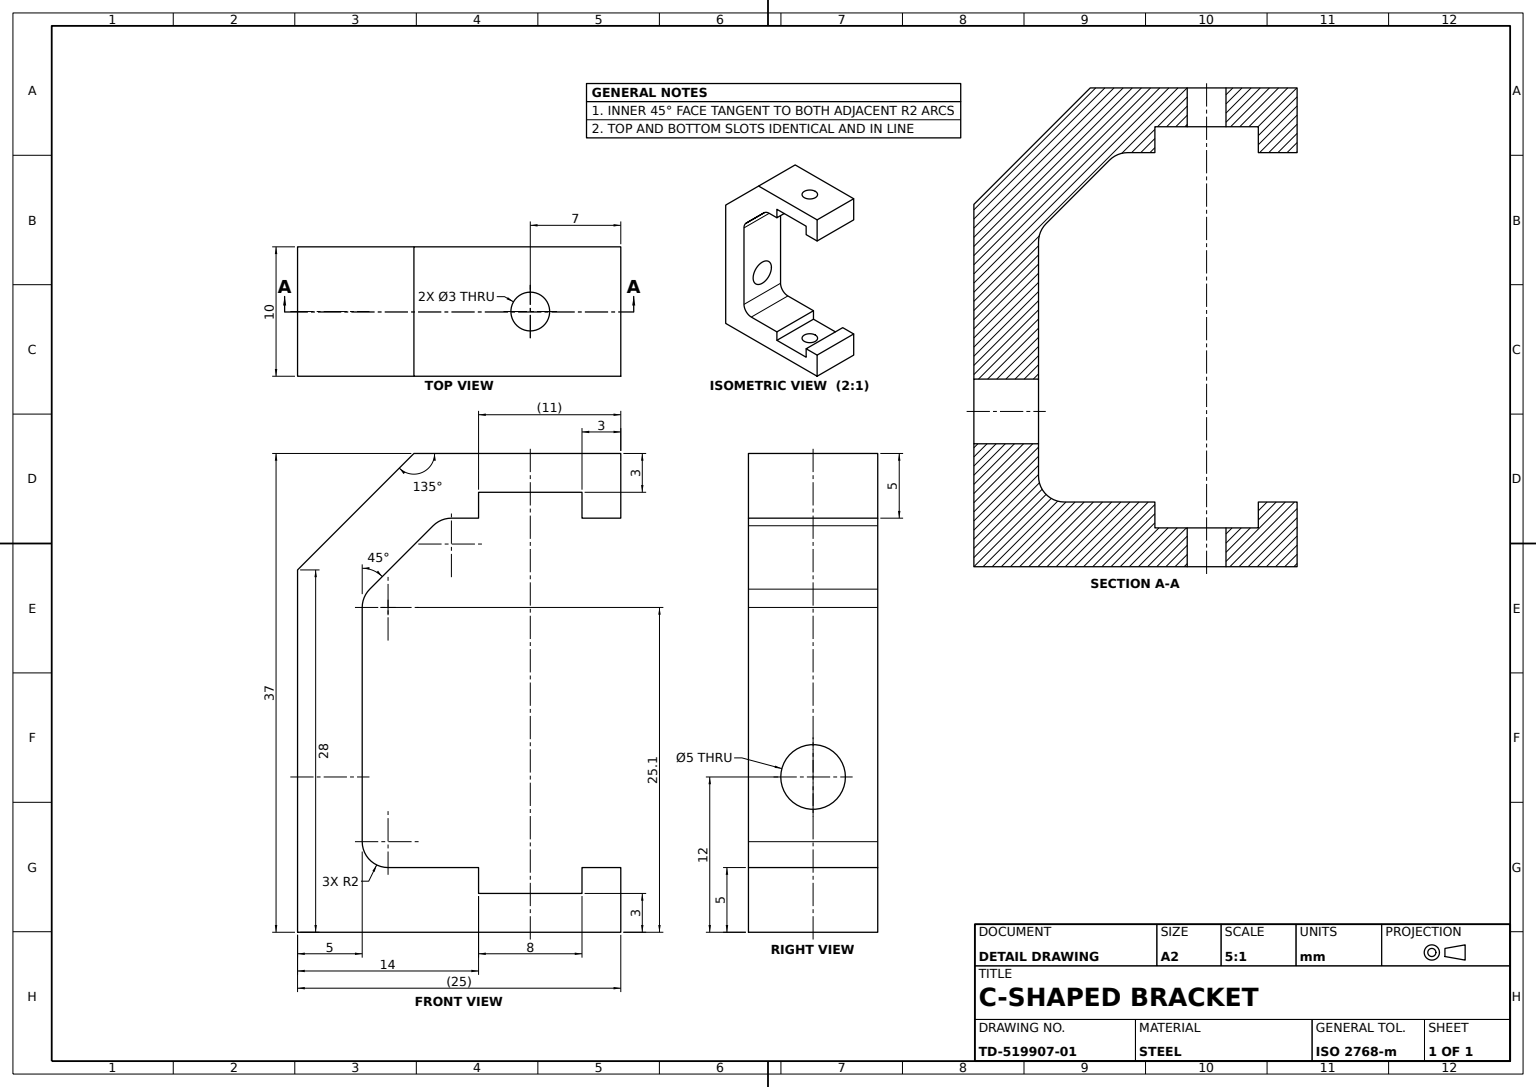
from build123d import *

# Parameters (mm, degrees)
C_CLIP_BODY_DEPTH      = 10
FLANGE_HOLE_1_SKETCH_R = 1.5
FLANGE_HOLE_1_3_DEPTH  = 100
FLANGE_HOLE_2_SKETCH_R = 1.5
FLANGE_HOLE_2_3_DEPTH  = 100
WEB_HOLE_SKETCH_R      = 2.5
WEB_HOLE_5_DEPTH       = 100


with BuildPart() as part:
    # C Clip Profile Sketch → C Clip Body (new body)
    with BuildSketch(Plane.XY):
        with BuildLine():
            Line((0, 0), (0, 28))
            Line((0, 28), (9, 37))
            Line((9, 37), (25, 37))
            Line((25, 37), (25, 32))
            Line((25, 32), (22, 32))
            Line((22, 32), (22, 34))
            Line((22, 34), (14, 34))
            Line((14, 34), (14, 32))
            Line((14, 32), (11.899494937, 32))
            ThreePointArc((11.899494937, 32), (11.134128072, 31.847759065), (10.485281374, 31.414213562))
            Line((10.485281374, 31.414213562), (5.585786438, 26.514718626))
            ThreePointArc((5.585786438, 26.514718626), (5.152240935, 25.865871928), (5, 25.100505063))
            Line((5, 25.100505063), (5, 7))
            ThreePointArc((5, 7), (5.585786438, 5.585786438), (7, 5))
            Line((7, 5), (14, 5))
            Line((14, 5), (14, 3))
            Line((14, 3), (22, 3))
            Line((22, 3), (22, 5))
            Line((22, 5), (25, 5))
            Line((25, 5), (25, 0))
            Line((25, 0), (0, 0))
        make_face()
    extrude(amount=C_CLIP_BODY_DEPTH)

    # Flange Hole 1 Sketch → Flange Hole 1 Ø3 (cut)
    with BuildSketch(Plane(origin=(0, 3, 0), x_dir=(1, 0, 0), z_dir=(0, 1, 0))):
        with Locations(Location((18, -5, 0), (0, 0, 270))):
            Circle(FLANGE_HOLE_1_SKETCH_R)
    extrude(amount=-FLANGE_HOLE_1_3_DEPTH, mode=Mode.SUBTRACT)

    # Flange Hole 2 Sketch → Flange Hole 2 Ø3 (cut)
    with BuildSketch(Plane(origin=(0, 37, 0), x_dir=(1, 0, 0), z_dir=(0, 1, 0))):
        with Locations(Location((18, -5, 0), (0, 0, 270))):
            Circle(FLANGE_HOLE_2_SKETCH_R)
    extrude(amount=-FLANGE_HOLE_2_3_DEPTH, mode=Mode.SUBTRACT)

    # Web Hole Sketch → Web Hole Ø5 (cut)
    with BuildSketch(Plane.ZY):
        with Locations((5, 12)):
            Circle(WEB_HOLE_SKETCH_R)
    extrude(amount=-WEB_HOLE_5_DEPTH, mode=Mode.SUBTRACT)


solid = part.part
